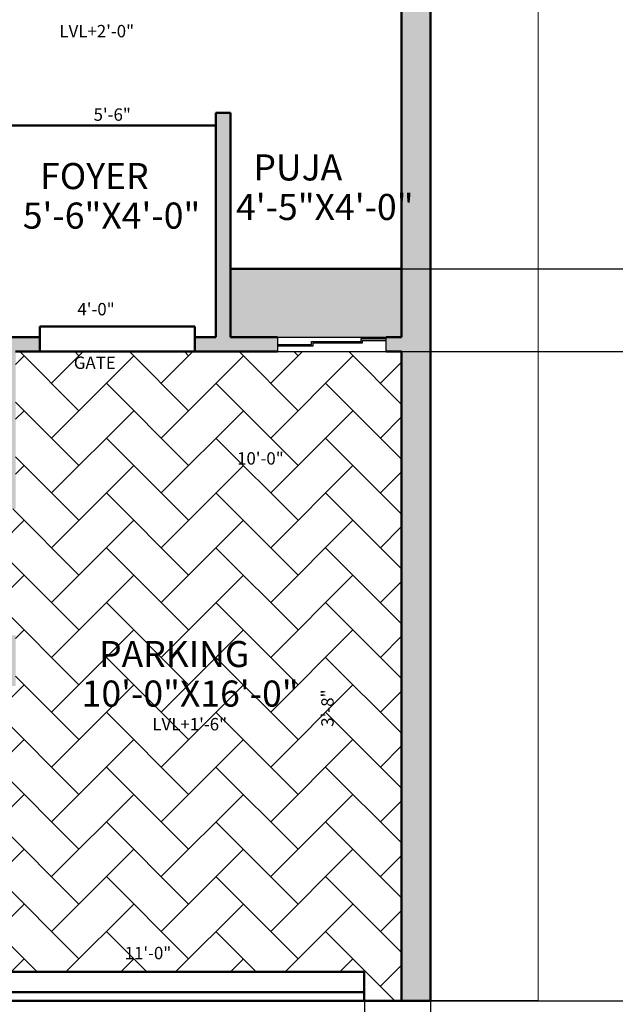
# Model space of a CAD drawing. Units: inches. Extents: x 1381 to 2246, y 1317 to 2168.
# Tile 4 of 15: x 1619 to 1804, y 1471 to 1776. Entities that reach past the tile are written whole.
import ezdxf

# ---------------------------------------------------------------- set-up
doc = ezdxf.new("R2010")
doc.units = ezdxf.units.IN
doc.header["$MEASUREMENT"] = 0
for name, color, linetype, lineweight in [('A-ANNO-DIMS', 2, 'Continuous', 18), ('A-ANNO-TEXT', 7, 'Continuous', 18), ('A-AREA-IDEN', 3, 'Continuous', 25), ('A-FLOR-PATT', 252, 'Continuous', 13), ('A-GLAZ', 4, 'Continuous', 25), ('A-WALL', 7, 'Continuous', 50), ('A-WALL-PATT', 8, 'Continuous', 13)]:
    doc.layers.add(name, color=color, linetype=linetype, lineweight=lineweight)
doc.styles.get("Standard").update_dxf_attribs({"font": 'arial.ttf'})
doc.dimstyles.get("Standard").update_dxf_attribs({"dimtxt": 7, "dimasz": 0.18, "dimexe": 0.18, "dimexo": 0.0625, "dimgap": 0.09, "dimtad": 0, "dimtih": 1, "dimtoh": 1, "dimdec": 1, "dimzin": 0, "dimdsep": 46, "dimlunit": 3, "dimtxsty": 'Standard', "dimcen": 0.09, "dimadec": 0, "dimazin": 0, "dimtfac": 1, "dimtdec": 1, "dimtofl": 0, "dimtmove": 0, "dimatfit": 3, "dimfxl": 1, "dimtolj": 1, "dimtzin": 0, "dimarcsym": 0})

# ---------------------------------------------------------------- blocks, each defined once
blk = doc.blocks.new('*D49')
at = {"layer": 'A-ANNO-DIMS', "color": 0, "lineweight": -2, "transparency": 16777216}
for p, q in [((1447.05, 1471.85), (1447.05, 1384.36)), ((1746.55, 1471.85), (1746.55, 1384.36)), ((1447.23, 1384.54), (1584.81, 1384.54)), ((1746.37, 1384.54), (1608.79, 1384.54))]:
    blk.add_line(p, q, dxfattribs=at)
at = {"layer": 'A-ANNO-DIMS', "color": 0, "transparency": 16777216}
for points in [[(1447.23, 1384.57), (1447.23, 1384.51), (1447.05, 1384.54)], [(1746.37, 1384.57), (1746.37, 1384.51), (1746.55, 1384.54)]]:
    blk.add_solid(points, dxfattribs=at)
at = {"layer": 'Defpoints', "color": 0, "transparency": 16777216}
for p in [(1447.05, 1471.92), (1746.55, 1471.92), (1746.55, 1384.54)]:
    blk.add_point(p, dxfattribs=at)
at = {"layer": 'A-ANNO-DIMS', "color": 0, "transparency": 16777216, "insert": (1596.8, 1384.54), "char_height": 7, "attachment_point": 5}
blk.add_mtext('\\A1;299.5', dxfattribs=at)
blk = doc.blocks.new('*D60')
at = {"layer": 'A-ANNO-DIMS', "color": 0, "lineweight": -2, "transparency": 16777216}
for p, q in [((1737.61, 1672.92), (1818.27, 1672.92)), ((1818.09, 1672.74), (1818.09, 1576.08)), ((1818.09, 1472.1), (1818.09, 1568.75)), ((1737.61, 1471.92), (1818.27, 1471.92))]:
    blk.add_line(p, q, dxfattribs=at)
at = {"layer": 'A-ANNO-DIMS', "color": 0, "transparency": 16777216}
for points in [[(1818.06, 1672.74), (1818.12, 1672.74), (1818.09, 1672.92)], [(1818.06, 1472.1), (1818.12, 1472.1), (1818.09, 1471.92)]]:
    blk.add_solid(points, dxfattribs=at)
at = {"layer": 'Defpoints', "color": 0, "transparency": 16777216}
for p in [(1737.55, 1672.92), (1818.09, 1672.92), (1737.55, 1471.92)]:
    blk.add_point(p, dxfattribs=at)
at = {"layer": 'A-ANNO-DIMS', "color": 0, "transparency": 16777216, "insert": (1818.09, 1572.42), "char_height": 7, "attachment_point": 5}
blk.add_mtext('\\A1;201', dxfattribs=at)
blk = doc.blocks.new('*D61')
at = {"layer": 'A-ANNO-DIMS', "color": 0, "lineweight": -2, "transparency": 16777216}
for p, q in [((1737.61, 1911.42), (1818.27, 1911.42)), ((1818.09, 1911.24), (1818.09, 1808.63)), ((1818.09, 1698.7), (1818.09, 1801.3)), ((1737.61, 1698.52), (1818.27, 1698.52))]:
    blk.add_line(p, q, dxfattribs=at)
at = {"layer": 'A-ANNO-DIMS', "color": 0, "transparency": 16777216}
for points in [[(1818.06, 1911.24), (1818.12, 1911.24), (1818.09, 1911.42)], [(1818.06, 1698.7), (1818.12, 1698.7), (1818.09, 1698.52)]]:
    blk.add_solid(points, dxfattribs=at)
at = {"layer": 'Defpoints', "color": 0, "transparency": 16777216}
for p in [(1737.55, 1911.42), (1818.09, 1911.42), (1737.55, 1698.52)]:
    blk.add_point(p, dxfattribs=at)
at = {"layer": 'A-ANNO-DIMS', "color": 0, "transparency": 16777216, "insert": (1818.09, 1804.97), "char_height": 7, "attachment_point": 5}
blk.add_mtext('\\A1;212.9', dxfattribs=at)
blk = doc.blocks.new('*D65')
at = {"layer": 'A-ANNO-DIMS', "color": 0, "lineweight": -2, "transparency": 16777216}
for p, q in [((1594.05, 1471.85), (1594.05, 1384.36)), ((1726.05, 1471.85), (1726.05, 1384.36)), ((1594.23, 1384.54), (1652.59, 1384.54)), ((1725.87, 1384.54), (1667.5, 1384.54))]:
    blk.add_line(p, q, dxfattribs=at)
at = {"layer": 'A-ANNO-DIMS', "color": 0, "transparency": 16777216}
for points in [[(1594.23, 1384.57), (1594.23, 1384.51), (1594.05, 1384.54)], [(1725.87, 1384.57), (1725.87, 1384.51), (1726.05, 1384.54)]]:
    blk.add_solid(points, dxfattribs=at)
at = {"layer": 'Defpoints', "color": 0, "transparency": 16777216}
for p in [(1594.05, 1471.92), (1726.05, 1471.92), (1726.05, 1384.54)]:
    blk.add_point(p, dxfattribs=at)
at = {"layer": 'A-ANNO-DIMS', "color": 0, "transparency": 16777216, "insert": (1660.05, 1384.54), "char_height": 7, "attachment_point": 5}
blk.add_mtext('\\A1;132', dxfattribs=at)

msp = doc.modelspace()

# ---------------------------------------------------------------- hatches: boundary and pattern name
at = {"layer": 'A-FLOR-PATT'}
h = msp.add_hatch(dxfattribs=at)
h.set_pattern_fill('AR-HBONE', color=256, scale=3)
h.paths.add_polyline_path([(1737.551, 1672.9163), (1732.8596, 1672.9163), (1699.1735, 1672.9163), (1618.051, 1672.9163), (1618.051, 1624.2465), (1613.551, 1624.2465), (1613.551, 1585.1257), (1618.051, 1585.1257), (1618.051, 1569.4163), (1609.051, 1569.4163), (1588.9723, 1569.4163), (1588.9723, 1480.9163), (1594.0453, 1480.9163), (1726.0453, 1480.9163), (1726.0453, 1471.9163), (1737.551, 1471.9163)])
at = {"layer": 'A-GLAZ'}
h = msp.add_hatch(color=256, dxfattribs=at)
h.dxf.hatch_style = 1
h.paths.add_polyline_path([(1456.051, 2083.9163), (1737.551, 2083.9163), (1737.551, 1677.4163), (1732.8596, 1677.4163), (1732.8596, 1672.9163), (1737.551, 1672.9163), (1737.551, 1471.9163), (1746.551, 1471.9163), (1746.551, 2092.9163), (1447.051, 2092.9163), (1447.051, 2083.9163), (1447.051, 1471.9163), (1488.6632, 1471.9163), (1488.6632, 1480.9163), (1456.051, 1480.9163), (1456.051, 1710.4163), (1517.1194, 1710.4163), (1517.1194, 1714.9163), (1491.551, 1714.9163), (1491.551, 1729.193), (1487.051, 1729.193), (1487.051, 1714.9163), (1456.051, 1714.9163)])
h.paths.add_polyline_path([(1622.551, 2035.4163), (1625.0954, 2035.4163), (1625.0954, 2039.9163), (1618.051, 2039.9163), (1618.051, 1915.9163), (1611.2353, 1915.9163), (1611.2353, 1911.4163), (1626.5102, 1911.4163), (1626.5102, 1915.9163), (1622.551, 1915.9163)], flags=17)
h.paths.add_polyline_path([(1737.551, 1915.9163), (1668.5102, 1915.9163), (1668.5102, 1911.4163), (1737.551, 1911.4163)], flags=17)
h.paths.add_polyline_path([(1682.2831, 2039.9163), (1655.8191, 2039.9163), (1655.8191, 2035.4163), (1682.2831, 2035.4163)], flags=17)
h.paths.add_polyline_path([(1737.551, 2039.9163), (1725.9636, 2039.9163), (1725.9636, 2035.4163), (1737.551, 2035.4163)], flags=17)
h.paths.add_polyline_path([(1684.2508, 1711.4667), (1740.8192, 1711.4667), (1740.8192, 1723.8346), (1684.2508, 1723.8346)], flags=25)
h = msp.add_hatch(color=256, dxfattribs=at)
h.dxf.hatch_style = 1
h.paths.add_polyline_path([(1478.9621, 1915.9163), (1456.051, 1915.9163), (1456.051, 1911.4163), (1478.9621, 1911.4163)])
h.paths.add_polyline_path([(1566.2107, 1915.9163), (1511.016, 1915.9163), (1511.016, 1911.4163), (1516.051, 1911.4163), (1516.051, 1779.4163), (1484.0852, 1779.4163), (1484.0852, 1774.9163), (1487.051, 1774.9163), (1487.051, 1755.1129), (1491.551, 1755.1129), (1491.551, 1774.9163), (1563.551, 1774.9163), (1563.551, 1770.3401), (1568.051, 1770.3401), (1568.051, 1779.4163), (1520.551, 1779.4163), (1520.551, 1911.4163), (1566.2107, 1911.4163)])
h.paths.add_polyline_path([(1568.051, 1734.7997), (1563.551, 1734.7997), (1563.551, 1714.9163), (1557.5961, 1714.9163), (1557.5961, 1710.4163), (1568.051, 1710.4163)])
h.paths.add_polyline_path([(1458.1653, 1779.4163), (1456.051, 1779.4163), (1456.051, 1774.9163), (1458.1653, 1774.9163)])
h.paths.add_polyline_path([(1684.551, 1746.8536), (1680.051, 1746.8536), (1680.051, 1677.4163), (1673.5117, 1677.4163), (1673.5117, 1672.9163), (1699.1735, 1672.9163), (1699.1735, 1677.4163), (1684.551, 1677.4163)])
h.paths.add_polyline_path([(1613.551, 1746.8536), (1609.051, 1746.8536), (1609.051, 1624.2465), (1618.051, 1624.2465), (1618.051, 1672.9163), (1625.5117, 1672.9163), (1625.5117, 1677.4163), (1613.551, 1677.4163)])
h.paths.add_polyline_path([(1618.051, 1585.1257), (1609.051, 1585.1257), (1609.051, 1569.4163), (1618.051, 1569.4163)])
h.paths.add_polyline_path([(1545.7088, 1578.4163), (1456.051, 1578.4163), (1456.051, 1569.4163), (1545.7088, 1569.4163)])
h.paths.add_polyline_path([(1594.0453, 1480.9163), (1536.6467, 1480.9163), (1536.6467, 1471.9163), (1594.0453, 1471.9163)])
h = msp.add_hatch(color=256, dxfattribs=at)
h.dxf.hatch_style = 1
h.paths.add_polyline_path([(1710.2123, 1675.6607), (1725.5171, 1675.6607), (1725.5171, 1676.3635), (1732.8596, 1676.3635), (1732.8596, 1676.9597), (1725.1121, 1676.9597), (1725.1121, 1676.0866), (1709.6793, 1676.0866), (1709.6793, 1675.1663), (1699.1735, 1675.1663), (1699.1735, 1674.7024), (1710.2123, 1674.7024)])
at = {"layer": 'A-WALL-PATT'}
h = msp.add_hatch(color=256, dxfattribs=at)
h.dxf.hatch_style = 1
h.paths.add_polyline_path([(1737.551, 1698.5169), (1684.551, 1698.5169), (1684.551, 1677.4163), (1699.1735, 1677.4163), (1732.8596, 1677.4163), (1737.551, 1677.4163)])

# ---------------------------------------------------------------- linework, layer by layer
at = {"layer": 'A-ANNO-DIMS'}
msp.add_line((1779.8404, 2092.9163), (1779.8404, 1471.9163), dxfattribs=at)
at = {"layer": 'A-GLAZ'}
for p, q in [((1699.1735, 1677.4163), (1699.1735, 1672.9163)), ((1699.1735, 1677.4163), (1732.8596, 1677.4163)), ((1725.1121, 1676.0866), (1725.1121, 1676.9597)), ((1725.1121, 1676.9597), (1732.8596, 1676.9597)), ((1732.8596, 1672.9163), (1732.8596, 1677.4163)), ((1699.1735, 1675.1663), (1709.6793, 1675.1663)), ((1699.1735, 1674.7024), (1710.2123, 1674.7024)), ((1709.6793, 1675.1663), (1709.6793, 1676.0866)), ((1709.6793, 1676.0866), (1725.1121, 1676.0866)), ((1710.2123, 1674.7024), (1710.2123, 1675.6607)), ((1710.2123, 1675.6607), (1725.5171, 1675.6607)), ((1725.5171, 1675.6607), (1725.5171, 1676.3635)), ((1725.5171, 1676.3635), (1732.8596, 1676.3635)), ((1699.1735, 1672.9163), (1732.8596, 1672.9163)), ((1779.8404, 1471.9163), (1746.551, 1471.9163))]:
    msp.add_line(p, q, dxfattribs=at)
at = {"layer": 'A-WALL'}
for p, q in [((1746.551, 2092.9163), (1746.551, 1471.9163)), ((1737.551, 2083.9163), (1737.551, 1677.4163)), ((1680.051, 1746.8536), (1680.051, 1677.4163)), ((1680.051, 1746.8536), (1684.551, 1746.8536)), ((1684.551, 1746.8536), (1684.551, 1677.4163)), ((1613.551, 1742.952), (1680.051, 1742.952)), ((1684.551, 1698.5169), (1737.551, 1698.5169)), ((1625.5117, 1672.9163), (1625.5117, 1680.6861)), ((1625.5117, 1680.6861), (1673.5117, 1680.6861)), ((1673.5117, 1680.6861), (1673.5117, 1672.9163)), ((1673.5117, 1680.6861), (1673.5117, 1680.6861)), ((1613.551, 1677.4163), (1625.5117, 1677.4163)), ((1673.5117, 1677.4163), (1680.051, 1677.4163)), ((1684.551, 1677.4163), (1699.1735, 1677.4163)), ((1732.8596, 1677.4163), (1737.551, 1677.4163)), ((1618.051, 1672.9163), (1699.1735, 1672.9163)), ((1732.8596, 1672.9163), (1737.551, 1672.9163)), ((1737.551, 1672.9163), (1737.551, 1471.9163)), ((1594.0453, 1480.9163), (1726.0453, 1480.9163)), ((1726.0453, 1471.9163), (1726.0453, 1480.9163)), ((1594.0453, 1474.6181), (1726.0453, 1474.6181)), ((1447.051, 1471.9163), (1746.551, 1471.9163))]:
    msp.add_line(p, q, dxfattribs=at)

# ---------------------------------------------------------------- texts
at = {"layer": 'A-ANNO-TEXT'}
for s, p in [('LVL+2\'-0"', (1631.6122, 1770.2214)), ('5\'-6"', (1642.1968, 1744.3872)), ('4\'-0"', (1637.1842, 1684.1577)), ('GATE', (1636.07, 1667.5678)), ('10\'-0"', (1686.6379, 1637.9554)), ('LVL+1\'-6"', (1660.4072, 1555.6668)), ('11\'-0"', (1651.8153, 1484.8192))]:
    msp.add_text(s, height=3.83139, dxfattribs=at).set_placement(p)
msp.add_text('3\'-8"', height=3.83139, rotation=90, dxfattribs=at).set_placement((1716.5436, 1556.7937))
at = {"layer": 'A-AREA-IDEN'}
for s, height, p in [('FOYER', 8.07451, (1625.6658, 1723.2343)), ('PUJA', 8.07451, (1691.7061, 1725.9053)), ('4\'-5"X4\'-0"', 8.074511, (1686.3121, 1713.6657)), ('5\'-6"X4\'-0"', 8.074511, (1620.2718, 1710.9947)), ('PARKING', 8.07451, (1643.8997, 1575.2653)), ('10\'-0"X16\'-0"', 8.074511, (1638.5057, 1563.0256))]:
    msp.add_text(s, height=height, dxfattribs=at).set_placement(p)

# ---------------------------------------------------------------- dimensions: what is measured, and where the dimension line sits
at = {"layer": 'A-ANNO-DIMS'}
for base, p1, p2, override, picture, middle in [((1818.0904, 1911.4163), (1737.551, 1698.5169), (1737.551, 1911.4163), {"dimdec": 1, "dimlfac": 1, "dimrnd": 0, "dimzin": 0, "dimdsep": 46, "dimlunit": 2}, '*D61', (1818.0904, 1804.9666)), ((1818.0904, 1672.9163), (1737.551, 1471.9163), (1737.551, 1672.9163), {"dimdec": 0, "dimlfac": 1, "dimrnd": 0, "dimzin": 0, "dimdsep": 46, "dimlunit": 2}, '*D60', (1818.0904, 1572.4163))]:
    dim = msp.add_linear_dim(base=base, p1=p1, p2=p2, angle=90, dimstyle='Standard', override=override, dxfattribs=at)
    dim.commit()
    dim.dimension.update_dxf_attribs({"geometry": picture, "text_midpoint": middle})
for base, p1, p2, override, picture, middle in [((1746.551, 1384.5407), (1447.051, 1471.9163), (1746.551, 1471.9163), {"dimdec": 1, "dimlfac": 1, "dimrnd": 0, "dimzin": 0, "dimdsep": 46, "dimlunit": 2}, '*D49', (1596.801, 1384.5407)), ((1726.0453, 1384.5407), (1594.0453, 1471.9163), (1726.0453, 1471.9163), {"dimdec": 0, "dimlfac": 1, "dimrnd": 0, "dimzin": 0, "dimdsep": 46, "dimlunit": 2}, '*D65', (1660.0453, 1384.5407))]:
    dim = msp.add_linear_dim(base=base, p1=p1, p2=p2, dimstyle='Standard', override=override, dxfattribs=at)
    dim.commit()
    dim.dimension.update_dxf_attribs({"geometry": picture, "text_midpoint": middle})

doc.saveas('drawing.dxf')
